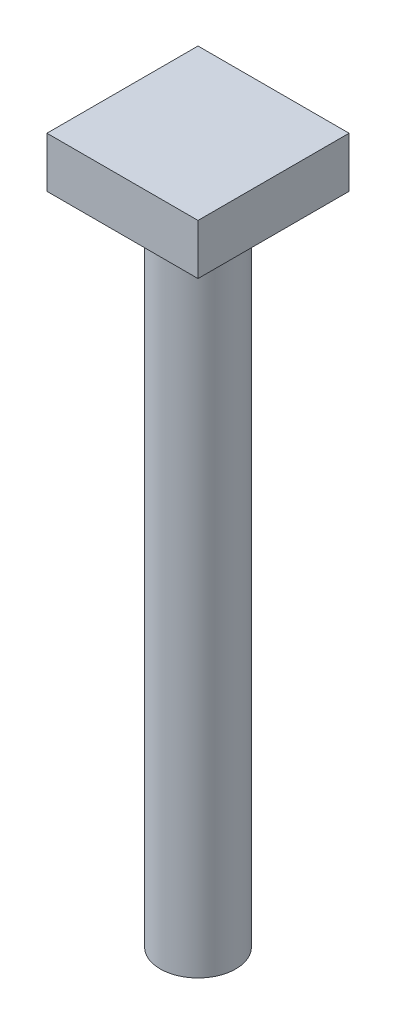
SolidWorks part; units mm, degrees
material "Plain Carbon Steel"
ref_plane "Front Plane" through (0, 0, 0) normal (0, 0, 1) x (1, 0, 0)
ref_plane "Top Plane" through (0, 0, 0) normal (0, 1, 0) x (1, 0, 0)
ref_plane "Right Plane" through (0, 0, 0) normal (1, 0, 0) x (0, 0, -1)
sketch "Head Profile 24x24" plane through (0, 0, 0) normal (0, 1, 0) x (1, 0, 0)
  line L1 (-12, 12) -> (12, 12)
  line L2 (-12, 12) -> (-12, -12)
  line L3 (-12, -12) -> (12, -12)
  line L4 (12, 12) -> (12, -12)
  line L5 (-12, 12) -> (12, -12) construction
  line L6 (-12, -12) -> (12, 12) construction
  point P0 (0, 0)
  dimension "D1" = 24
  dimension "D2" = 24
extrude "Square Head 24x24x8" add sketch "Head Profile 24x24" along normal blind 8
sketch "Shank Profile Ø12" plane through (0, 0, 0) normal (0, -1, 0) x (1, 0, 0)
  circle A0 centre (0, 0) radius 6
  dimension "D1" = 12
extrude "Shank Ø12x104" add sketch "Shank Profile Ø12" along normal blind 104
